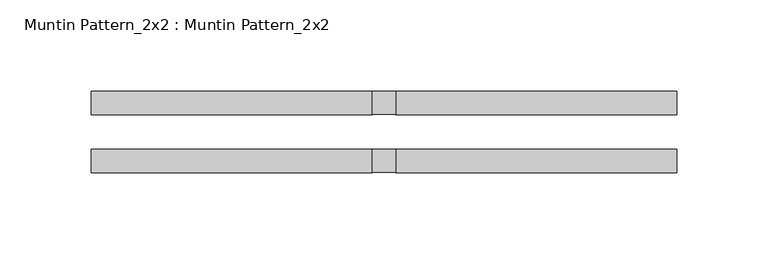
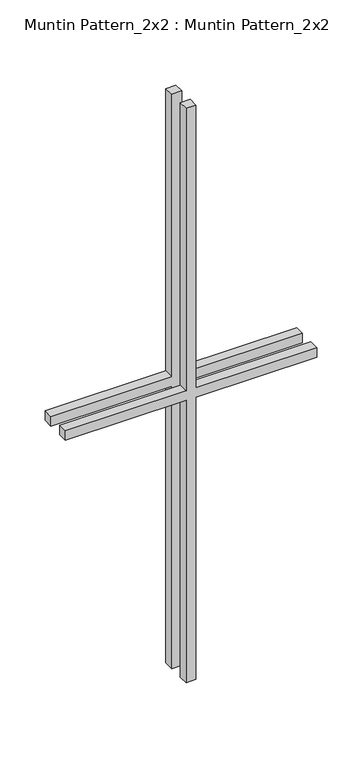
"""IFC4 building model written with IfcOpenShell, lengths in millimetres: proxy geometry, Muntin Pattern_2x2 : Muntin Pattern_2x2."""

from ifc_helpers import new_model, si_unit, frame, origin, place, context, project, spatial, polyline, outline, extrude, source, transform, mapped, element, save


def muntin_pattern_2x2_muntin_pattern_2x2_d1c6e638(model_context):
    return source(origin(), model_context, "Body", "SweptSolid", [
        extrude(outline(polyline([(393.7, -6.35), (393.7, -160.3375), (381.0, -160.3375), (381.0, -6.35), (0.0, -6.35), (0.0, 6.35), (381.0, 6.35), (381.0, 160.3375), (393.7, 160.3375), (393.7, 6.35), (774.7, 6.35), (774.7, -6.35), (393.7, -6.35)])), frame((0.0, 9.525, 0.0), z_axis=(0.0, 1.0, 0.0), x_axis=(0.0, 0.0, 1.0)), (0.0, 0.0, 1.0), 12.7),
        extrude(outline(polyline([(393.7, -6.35), (393.7, -160.3375), (381.0, -160.3375), (381.0, -6.35), (0.0, -6.35), (0.0, 6.35), (381.0, 6.35), (381.0, 160.3375), (393.7, 160.3375), (393.7, 6.35), (774.7, 6.35), (774.7, -6.35), (393.7, -6.35)])), frame((0.0, -22.225, 0.0), z_axis=(0.0, 1.0, 0.0), x_axis=(0.0, 0.0, 1.0)), (0.0, 0.0, 1.0), 12.7),
    ])


if __name__ == "__main__":
    model = new_model("IFC4")
    model_context = context("Model", 3, world=origin())
    ifc_project = project(units=[si_unit("LENGTHUNIT", "METRE", prefix="MILLI")], contexts=[model_context])
    site = spatial("IfcSite", under=ifc_project)
    building = spatial("IfcBuilding", under=site)
    placement = place(None, origin())
    muntin_pattern_2x2_muntin_pattern_2x2_shape = muntin_pattern_2x2_muntin_pattern_2x2_d1c6e638(model_context)
    element("IfcBuildingElementProxy", 1, Name="Muntin Pattern_2x2 : Muntin Pattern_2x2", ObjectType="Muntin Pattern_2x2 : Muntin Pattern_2x2", at=placement, inside=building, context=model_context, shape_type="MappedRepresentation", body=[
        mapped(muntin_pattern_2x2_muntin_pattern_2x2_shape, transform((0.0, 0.0, 0.0), x_axis=(1.0, 0.0, 0.0), y_axis=(0.0, 1.0, 0.0), z_axis=(0.0, 0.0, 1.0))),
    ])
    save(model, "model.ifc")

# Revit data of these elements
# Type "Muntin Pattern_2x2 : Muntin Pattern_2x2"
#   Width [instance default] = 4' - 0"
#   Thickness = 0' - 0 1/2"
#   Height [instance default] = 4' - 0"
#   Distance = 0' - 0 3/4"
#   Interior Material [instance default] = none
#   Exterior Material [instance default] = none
#   Default Elevation = 0
# Element 1 (IfcBuildingElementProxy, "Muntin Pattern_2x2 : Muntin Pattern_2x2")
#   Width = 1' - 0 5/8"
#   Height = 2' - 6 1/2"
#   Interior Material = Wood - Stained
#   Materials on its faces: "Wood - Stained"
# Materials
#   "Wood - Stained": class "Wood", colour RGB 224 178 126, transparency 0, Cost = 0
